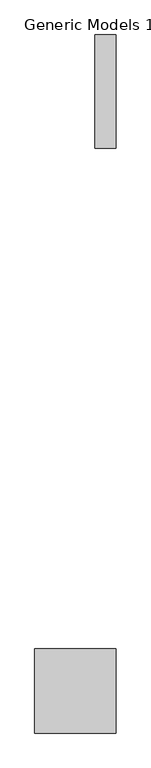
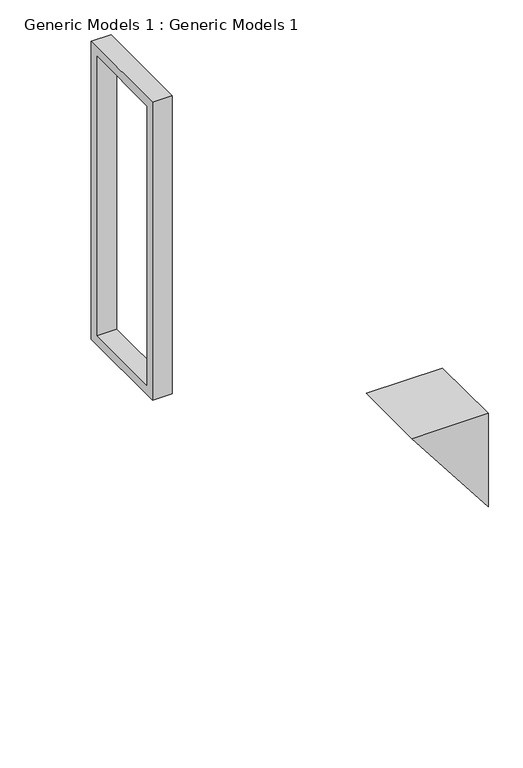
"""IFC4 building model written with IfcOpenShell, lengths in millimetres: proxy geometry, Generic Models 1 : Generic Models 1."""

from ifc_helpers import new_model, si_unit, frame, origin, place, context, project, spatial, polyline, outline, extrude, faceted_brep, source, transform, mapped, element, save


def generic_models_1_generic_models_1_7359c5b6(model_context):
    return source(origin(), model_context, "Body", "SolidModel", [
        faceted_brep([(-15539.3231107, -3758.4534819, 3962.4), (-15539.3231107, -3758.4534819, 5486.4), (-15539.3231107, -4977.6534819, 5486.4), (-15539.3231107, -4977.6534819, 3962.4), (-15539.3231107, -3910.8534819, 4114.8), (-15539.3231107, -4825.2534819, 4114.8), (-15539.3231107, -4825.2534819, 5334.0), (-15539.3231107, -3910.8534819, 5334.0), (-16596.8434996, -3910.8534819, 5334.0), (-15656.8253761, -3910.8534819, 4114.8), (-16596.8434996, -4825.2534819, 5334.0), (-15656.8253761, -4825.2534819, 4114.8), (-16714.3457651, -4977.6534819, 5486.4), (-16714.3457651, -3758.4534819, 5486.4)], [[[0, 1, 2, 3], [4, 5, 6, 7]], [[4, 7, 8, 9]], [[7, 6, 10, 8]], [[6, 5, 11, 10]], [[5, 4, 9, 11]], [[3, 2, 12]], [[2, 1, 13, 12]], [[1, 0, 13]], [[0, 3, 12, 13], [9, 8, 10, 11]]]),
        extrude(outline(polyline([(5112.4965181, 682.6676291), (3474.1965181, 682.6676291), (3474.1965181, 5543.55), (5112.4965181, 5543.55), (5112.4965181, 682.6676291)]), holes=[polyline([(4960.0965181, 835.0676291), (4960.0965181, 5391.15), (3626.5965181, 5391.15), (3626.5965181, 835.0676291), (4960.0965181, 835.0676291)])]), frame((-15844.1231107, 0.0, 0.0), z_axis=(1.0, 0.0, 0.0), x_axis=(0.0, 1.0, 0.0)), (0.0, 0.0, 1.0), 304.8),
    ])


if __name__ == "__main__":
    model = new_model("IFC4")
    model_context = context("Model", 3, world=origin())
    ifc_project = project(units=[si_unit("LENGTHUNIT", "METRE", prefix="MILLI")], contexts=[model_context])
    site = spatial("IfcSite", under=ifc_project)
    building = spatial("IfcBuilding", under=site)
    placement = place(None, origin())
    generic_models_1_generic_models_1_shape = generic_models_1_generic_models_1_7359c5b6(model_context)
    element("IfcBuildingElementProxy", 1, Name="Generic Models 1 : Generic Models 1", ObjectType="Generic Models 1 : Generic Models 1", at=placement, inside=building, context=model_context, shape_type="MappedRepresentation", body=[
        mapped(generic_models_1_generic_models_1_shape, transform((0.0, 0.0, 0.0), x_axis=(1.0, 0.0, 0.0), y_axis=(0.0, 1.0, 0.0), z_axis=(0.0, 0.0, 1.0))),
    ])
    save(model, "model.ifc")
